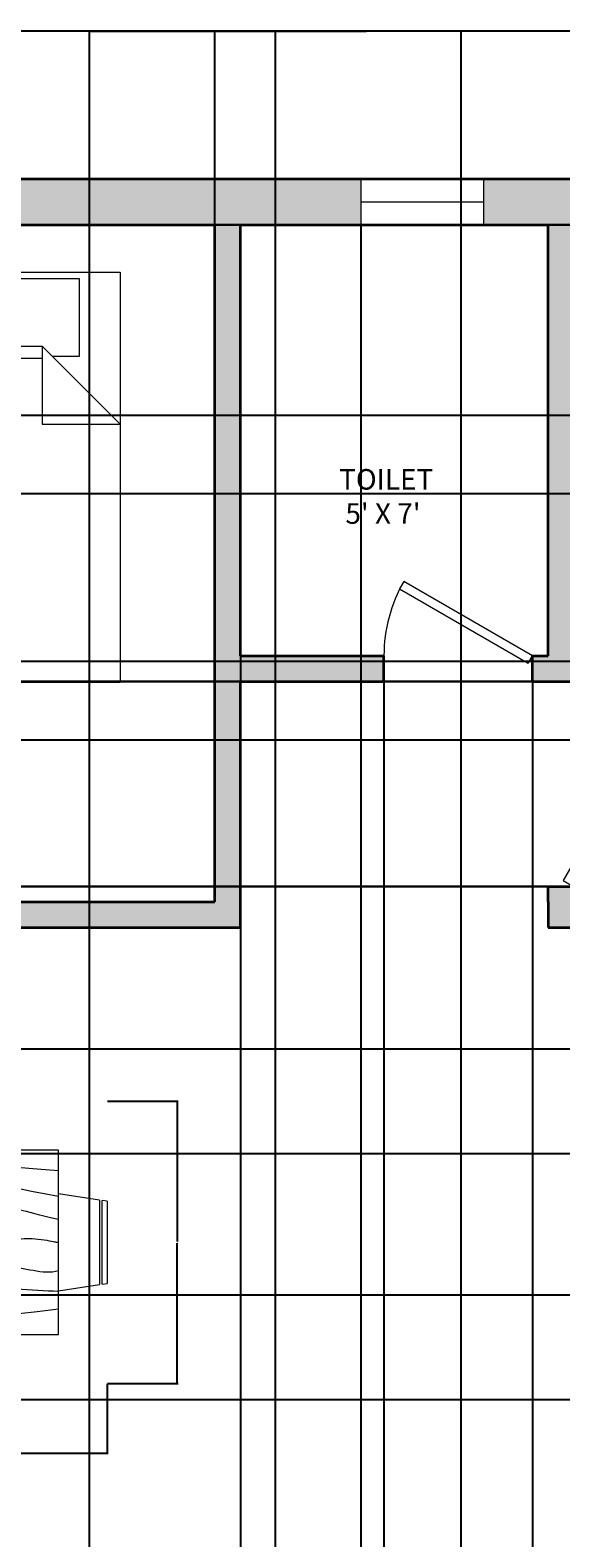
# Model space of a CAD drawing. Units: inches. Extents: x -28 to 649, y -11 to 509.
# Tile 6 of 7: x 346 to 450, y 215 to 509. Entities that reach past the tile are written whole.
import ezdxf

# ---------------------------------------------------------------- set-up
doc = ezdxf.new("R2010")
doc.units = ezdxf.units.IN
doc.header["$MEASUREMENT"] = 0
for name, color, linetype, lineweight in [('A-ANNO-DIMS', 2, 'Continuous', 18), ('A-AREA-IDEN', 18, 'Continuous', 18), ('A-WALL', 7, 'Continuous', 35), ('A-WALL-PATT', 251, 'Continuous', 13), ('doors', 40, 'Continuous', 20), ('furniture', 220, 'Continuous', 18), ('window', 30, 'Continuous', 18)]:
    doc.layers.add(name, color=color, linetype=linetype, lineweight=lineweight)
doc.styles.get("Standard").update_dxf_attribs({"font": 'arial.ttf'})
doc.dimstyles.get("Standard").update_dxf_attribs({"dimtxt": 0.18, "dimasz": 0.18, "dimexe": 0.18, "dimexo": 0.0625, "dimgap": 0.09, "dimtad": 0, "dimtih": 1, "dimtoh": 1, "dimdec": 4, "dimzin": 0, "dimdsep": 46, "dimtxsty": 'Standard', "dimcen": 0.09, "dimadec": 0, "dimazin": 0, "dimtfac": 1, "dimtdec": 4, "dimtofl": 0, "dimtmove": 0, "dimatfit": 3, "dimfxl": 1, "dimtolj": 1, "dimtzin": 0, "dimarcsym": 0})

# ---------------------------------------------------------------- blocks, each defined once
blk = doc.blocks.new('*U10')
for p, q in [((0, 0), (0, 100)), ((750, 0), (750, 100))]:
    blk.add_line(p, q)
blk.add_lwpolyline([(0, 0), (649.5, -375), (671.4, -337.1), (21.9, 37.9)], close=True)
blk.add_arc((0, 0), 750, 330, 0)
blk = doc.blocks.new('Dining Set - 36 x 72 in.')
for p, q in [((-22, 27.5), (-22.1562, 26.50042)), ((-5.8416, 26.5), (-22.1534, 26.5)), ((-22, 27.5), (-6, 27.5)), ((-5.8437, 26.49966), (-6, 27.5)), ((6, 27.5), (5.8438, 26.50042)), ((22.1584, 26.5), (5.8466, 26.5)), ((6, 27.5), (22, 27.5)), ((22.1563, 26.49966), (22, 27.5)), ((-22.2343, 26.00059), (-23.4847, 17.99762)), ((-22.2304, 26), (-5.7608, 26)), ((-4.5152, 17.99762), (-5.7655, 25.99926)), ((5.7657, 26.00059), (4.5153, 17.99762)), ((5.7696, 26), (22.2392, 26)), ((23.4848, 17.99762), (22.2345, 25.99926)), ((36, 18), (-36, 18)), ((-36, 18), (-36, -18)), ((36, -18), (36, 18)), ((-44.0006, 8.23428), (-35.9976, 9.48474)), ((44.0006, 8.23428), (35.9976, 9.48474)), ((-45.5, 8), (-44.5004, 8.15617)), ((-45.5, 8), (-45.5, -8)), ((-44.5, -8.15843), (-44.5, 8.15338)), ((-44, 8.23041), (-44, -8.23915)), ((44, 8.23041), (44, -8.23915)), ((44.5, -8.15843), (44.5, 8.15338)), ((45.5, 8), (44.5005, 8.15617)), ((45.5, 8), (45.5, -8)), ((-44.4997, -8.15631), (-45.5, -8)), ((-35.9976, -9.48476), (-43.9993, -8.2345)), ((35.9976, -9.48476), (43.9993, -8.2345)), ((44.4997, -8.15631), (45.5, -8)), ((-36, -18), (36, -18)), ((-22.2343, -26.0006), (-23.4847, -17.99762)), ((-4.5152, -17.99762), (-5.7655, -25.99928)), ((5.7657, -26.0006), (4.5153, -17.99762)), ((23.4848, -17.99762), (22.2345, -25.99928)), ((-22.2304, -26), (-5.7608, -26)), ((5.7696, -26), (22.2392, -26)), ((-22, -27.5), (-22.1562, -26.50044)), ((-5.8416, -26.5), (-22.1534, -26.5)), ((-22, -27.5), (-6, -27.5)), ((-5.8437, -26.49967), (-6, -27.5)), ((6, -27.5), (5.8438, -26.50044)), ((22.1584, -26.5), (5.8466, -26.5)), ((6, -27.5), (22, -27.5)), ((22.1563, -26.49967), (22, -27.5))]:
    blk.add_line(p, q)
for points in [[(-36, 15), (-31.1772, 14.97754), (-26.8079, 14.91406), (-22.8538, 14.81543), (-19.276, 14.6875), (-16.0362, 14.53613), (-13.0957, 14.36718), (-10.4159, 14.18652), (-7.9583, 14), (-5.6904, 13.81315), (-3.6035, 13.63021), (-1.6954, 13.45508), (0.0365, 13.29166), (1.5945, 13.14388), (2.9811, 13.01562), (4.1988, 12.9108), (5.25, 12.83333), (6.1393, 12.78613), (6.8802, 12.76823), (7.4883, 12.77767), (7.9792, 12.8125), (8.3685, 12.87077), (8.6719, 12.95052), (8.9049, 13.0498), (9.0833, 13.16666), (9.2205, 13.29899), (9.3216, 13.44401), (9.3895, 13.59879), (9.4271, 13.76041), (9.4373, 13.92594), (9.4232, 14.09245), (9.3875, 14.257), (9.3333, 14.41666), (9.2638, 14.56917), (9.1836, 14.71484), (9.0975, 14.85465), (9.0104, 14.98958), (8.9272, 15.1206), (8.8529, 15.2487), (8.7922, 15.37483), (8.75, 15.5), (8.7305, 15.62467), (8.7344, 15.74739), (8.7617, 15.86621), (8.8125, 15.97916), (8.8867, 16.08431), (8.9844, 16.17968), (9.1055, 16.26334), (9.25, 16.33333), (9.4189, 16.38802), (9.6172, 16.42708), (9.8506, 16.45052), (10.125, 16.45833), (10.4463, 16.45052), (10.8203, 16.42708), (11.2529, 16.38802), (11.75, 16.33333), (12.3184, 16.26318), (12.9694, 16.17838), (13.7151, 16.07991), (14.5677, 15.96875), (15.5395, 15.84586), (16.6426, 15.71224), (17.8893, 15.56884), (19.2917, 15.41666), (20.859, 15.25667), (22.5879, 15.08984), (24.4721, 14.91715), (26.5052, 14.73958), (28.6809, 14.5581), (30.9929, 14.3737), (33.4347, 14.18733), (36, 14)], [(-36, 10), (-28.9766, 10.14274), (-23.1725, 10.20442), (-18.4241, 10.19775), (-14.5677, 10.13541), (-11.4399, 10.03011), (-8.877, 9.89453), (-6.7154, 9.74137), (-4.7917, 9.58333), (-2.9698, 9.43082), (-1.2246, 9.28515), (0.4415, 9.14534), (2.026, 9.01041), (3.5266, 8.87939), (4.9408, 8.7513), (6.266, 8.62516), (7.5, 8.5), (8.6411, 8.37549), (9.6914, 8.2539), (10.6538, 8.13818), (11.5312, 8.03125), (12.3267, 7.93603), (13.043, 7.85547), (13.6831, 7.79248), (14.25, 7.75), (14.7471, 7.7303), (15.1797, 7.73307), (15.5537, 7.75732), (15.875, 7.80208), (16.1494, 7.86637), (16.3828, 7.94922), (16.5811, 8.04964), (16.75, 8.16666), (16.8944, 8.29915), (17.0143, 8.44531), (17.1089, 8.60319), (17.1771, 8.77083), (17.218, 8.94629), (17.2305, 9.1276), (17.2137, 9.31282), (17.1667, 9.5), (17.0895, 9.6875), (16.987, 9.875), (16.8649, 10.0625), (16.7292, 10.25), (16.5856, 10.4375), (16.4401, 10.625), (16.2985, 10.8125), (16.1667, 11), (16.05, 11.18733), (15.9518, 11.3737), (15.8752, 11.5581), (15.8229, 11.73958), (15.798, 11.91715), (15.8034, 12.08984), (15.842, 12.25667), (15.9167, 12.41666), (16.0295, 12.56836), (16.1784, 12.70833), (16.3605, 12.83268), (16.5729, 12.9375), (16.8127, 13.01888), (17.0768, 13.07291), (17.3625, 13.0957), (17.6667, 13.08333), (17.9894, 13.03312), (18.3418, 12.94726), (18.7382, 12.82918), (19.1927, 12.68229), (19.7195, 12.51001), (20.3327, 12.31575), (21.0465, 12.10294), (21.875, 11.875), (22.8357, 11.63354), (23.959, 11.37304), (25.2786, 11.08618), (26.8282, 10.76562), (28.6414, 10.40405), (30.752, 9.99414), (33.1936, 9.52856), (36, 9)], [(-36, 5.5), (-30.7157, 5.3348), (-26.069, 5.20963), (-21.9946, 5.11767), (-18.4271, 5.05208), (-15.3009, 5.00602), (-12.5508, 4.97265), (-10.1112, 4.94515), (-7.9167, 4.91666), (-5.909, 4.88167), (-4.0586, 4.83984), (-2.3429, 4.79215), (-0.7396, 4.73958), (0.7739, 4.6831), (2.22, 4.6237), (3.6213, 4.56233), (5, 4.5), (6.373, 4.43782), (7.7344, 4.3776), (9.0723, 4.32129), (10.375, 4.27083), (11.6309, 4.22819), (12.8281, 4.19531), (13.9551, 4.17415), (15, 4.16666), (15.954, 4.17448), (16.819, 4.19791), (17.6001, 4.23698), (18.3021, 4.29166), (18.9299, 4.36198), (19.4883, 4.44791), (19.9823, 4.54948), (20.4167, 4.66666), (20.7969, 4.79899), (21.1302, 4.94401), (21.4245, 5.09879), (21.6875, 5.26041), (21.9271, 5.42594), (22.1511, 5.59245), (22.3672, 5.757), (22.5834, 5.91666), (22.8065, 6.06868), (23.0404, 6.21093), (23.2879, 6.34147), (23.5521, 6.45833), (23.8358, 6.55957), (24.142, 6.64323), (24.4735, 6.70735), (24.8334, 6.75), (25.2235, 6.76969), (25.642, 6.76692), (26.0858, 6.74267), (26.5521, 6.69791), (27.0379, 6.63362), (27.5404, 6.55078), (28.0565, 6.45036), (28.5834, 6.33333), (29.1242, 6.19987), (29.7071, 6.04687), (30.3661, 5.87044), (31.1354, 5.66666), (32.0493, 5.43164), (33.142, 5.16146), (34.4475, 4.85221), (36, 4.5)], [(-36, -1), (-30.7915, -0.6591), (-26.0195, -0.38216), (-21.6519, -0.16284), (-17.6563, 0.00521), (-14.0005, 0.12833), (-10.6523, 0.21289), (-7.5796, 0.26522), (-4.75, 0.29166), (-2.134, 0.29793), (0.2878, 0.28711), (2.5317, 0.26163), (4.6146, 0.22396), (6.5529, 0.17651), (8.3633, 0.12174), (10.0623, 0.06209), (11.6667, 0), (13.1899, -0.06201), (14.6341, -0.1211), (15.9982, -0.17432), (17.2813, -0.21875), (18.4823, -0.25147), (19.6003, -0.26953), (20.6343, -0.27002), (21.5834, -0.25), (22.4481, -0.20768), (23.2357, -0.14584), (23.9549, -0.06836), (24.6146, 0.02083), (25.2235, 0.11784), (25.7904, 0.21875), (26.3241, 0.31966), (26.8334, 0.41666), (27.3265, 0.50618), (27.8099, 0.58593), (28.2894, 0.65397), (28.7709, 0.70833), (29.2601, 0.74707), (29.763, 0.76823), (30.2855, 0.76985), (30.8334, 0.75), (31.4088, 0.70784), (31.9994, 0.64713), (32.589, 0.57275), (33.1615, 0.48958), (33.7008, 0.4025), (34.1908, 0.3164), (34.6153, 0.23616), (34.9584, 0.16666), (35.2099, 0.11165), (35.3848, 0.07031), (35.504, 0.04069), (35.5886, 0.02083), (35.6594, 0.00879), (35.7377, 0.0026), (35.8442, 0.00032), (36, 0)], [(-36, -6.5), (-27.1843, -6.31267), (-20.084, -6.1263), (-14.469, -5.9419), (-10.1094, -5.76042), (-6.7752, -5.58285), (-4.2363, -5.41016), (-2.2629, -5.24333), (-0.625, -5.08334), (0.8708, -4.93099), (2.2715, -4.78646), (3.5872, -4.64974), (4.8281, -4.52084), (6.0046, -4.39974), (7.127, -4.28646), (8.2053, -4.18099), (9.25, -4.08334), (10.2705, -3.99382), (11.2734, -3.91407), (12.2647, -3.84603), (13.25, -3.79167), (14.2354, -3.75293), (15.2266, -3.73177), (16.2295, -3.73015), (17.25, -3.75), (18.2912, -3.79248), (19.3451, -3.85547), (20.4009, -3.93604), (21.4479, -4.03125), (22.4754, -4.13819), (23.4727, -4.25391), (24.4289, -4.37549), (25.3334, -4.5), (26.1785, -4.62492), (26.9694, -4.74935), (27.7145, -4.87281), (28.4219, -4.99479), (29.1, -5.11483), (29.7572, -5.23242), (30.4016, -5.34709), (31.0417, -5.45834), (31.6837, -5.56437), (32.3262, -5.65821), (32.9658, -5.73153), (33.599, -5.77604), (34.2224, -5.78345), (34.8327, -5.74545), (35.4264, -5.65373), (36, -5.5)], [(-36, -10), (-26.4022, -9.81299), (-18.4675, -9.62891), (-11.9839, -9.45069), (-6.7396, -9.28125), (-2.5226, -9.12354), (0.8789, -8.98047), (3.6769, -8.85498), (6.0833, -8.75), (8.2767, -8.66765), (10.3021, -8.60677), (12.1712, -8.56543), (13.8958, -8.54167), (15.4876, -8.53353), (16.9583, -8.53907), (18.3197, -8.55632), (19.5834, -8.58334), (20.7616, -8.61841), (21.8685, -8.66081), (22.9188, -8.71004), (23.9271, -8.76563), (24.9081, -8.82707), (25.8763, -8.89388), (26.8465, -8.96558), (27.8334, -9.04167), (28.8474, -9.12118), (29.8828, -9.20117), (30.93, -9.27824), (31.9792, -9.34896), (33.0205, -9.40991), (34.0443, -9.45768), (35.0407, -9.48885), (36, -9.5)], [(-36, -14.5), (-30.0881, -14.33513), (-25.0332, -14.21224), (-20.7312, -14.12647), (-17.0781, -14.07292), (-13.97, -14.04671), (-11.3027, -14.04297), (-8.9724, -14.05681), (-6.875, -14.08334), (-4.9224, -14.11833), (-3.0905, -14.16016), (-1.3709, -14.20785), (0.2448, -14.26042), (1.7647, -14.3169), (3.1973, -14.3763), (4.5507, -14.43767), (5.8333, -14.5), (7.0554, -14.5621), (8.235, -14.62175), (9.3922, -14.67652), (10.5469, -14.72396), (11.7192, -14.76164), (12.929, -14.78711), (14.1965, -14.79794), (15.5417, -14.79167), (16.9933, -14.76424), (18.6152, -14.70508), (20.4804, -14.60197), (22.6615, -14.44271), (25.2312, -14.21509), (28.2624, -13.9069), (31.8277, -13.50594), (36, -13)]]:
    blk.add_lwpolyline(points)
blk = doc.blocks.new('Bed - Queen')
for p, q in [((0, -80.00003), (0, 0)), ((0, 0), (59.99999, 0)), ((59.99999, 0), (59.99999, -80.00003)), ((7.99999, -1.2), (28.79998, -1.2)), ((7.99999, -14.4), (7.99999, -1.2)), ((28.79998, -1.2), (28.79998, -14.4)), ((31.19999, -1.2), (51.99999, -1.2)), ((31.19999, -14.4), (31.19999, -1.2)), ((51.99999, -1.2), (51.99999, -16.4)), ((0, -14.4), (44.8, -14.4)), ((59.99999, -29.6), (44.8, -14.4)), ((44.8, -14.4), (44.8, -29.6)), ((44.8, -16.8), (0, -16.8)), ((51.99999, -16.4), (46.79936, -16.4)), ((44.8, -29.6), (59.99999, -29.6)), ((59.99999, -80.00003), (0, -80.00003))]:
    blk.add_line(p, q)
blk = doc.blocks.new('WIN-24x9')
for p, q in [((0, 9), (0, 0)), ((24, 9), (0, 9)), ((0, 9), (0, 4.5)), ((24, 0), (24, 9)), ((0, 4.5), (24, 4.5)), ((0, 0), (24, 0))]:
    blk.add_line(p, q)
blk = doc.blocks.new('*D28')
at = {"layer": 'A-ANNO-DIMS', "color": 0, "lineweight": -2, "transparency": 16777216}
for p, q in [((270.49, 245), (270.49, 231.23)), ((361.49, 245), (361.49, 231.23)), ((270.67, 231.41), (315.04, 231.41)), ((361.31, 231.41), (316.94, 231.41))]:
    blk.add_line(p, q, dxfattribs=at)
at = {"layer": 'A-ANNO-DIMS', "color": 0, "transparency": 16777216}
for points in [[(270.67, 231.44), (270.67, 231.38), (270.49, 231.41)], [(361.31, 231.44), (361.31, 231.38), (361.49, 231.41)]]:
    blk.add_solid(points, dxfattribs=at)
at = {"layer": 'Defpoints', "color": 0, "transparency": 16777216}
for p in [(270.49, 245.06), (361.49, 245.06), (361.49, 231.41)]:
    blk.add_point(p, dxfattribs=at)
at = {"layer": 'A-ANNO-DIMS', "color": 0, "transparency": 16777216, "insert": (315.99, 231.41), "char_height": 0.18, "attachment_point": 5}
blk.add_mtext('\\A1;DINING SET 91', dxfattribs=at)
blk = doc.blocks.new('*D29')
at = {"layer": 'A-ANNO-DIMS', "color": 0, "lineweight": -2, "transparency": 16777216}
for p, q in [((361.55, 300.06), (375.32, 300.06)), ((375.14, 299.88), (375.14, 272.75)), ((375.14, 245.24), (375.14, 272.38)), ((361.55, 245.06), (375.32, 245.06))]:
    blk.add_line(p, q, dxfattribs=at)
at = {"layer": 'A-ANNO-DIMS', "color": 0, "transparency": 16777216}
for points in [[(375.11, 299.88), (375.17, 299.88), (375.14, 300.06)], [(375.11, 245.24), (375.17, 245.24), (375.14, 245.06)]]:
    blk.add_solid(points, dxfattribs=at)
at = {"layer": 'Defpoints', "color": 0, "transparency": 16777216}
for p in [(361.49, 300.06), (375.14, 300.06), (361.49, 245.06)]:
    blk.add_point(p, dxfattribs=at)
at = {"layer": 'A-ANNO-DIMS', "color": 0, "transparency": 16777216, "insert": (375.14, 272.56), "char_height": 0.18, "attachment_point": 5}
blk.add_mtext('\\A1;55', dxfattribs=at)
blk = doc.blocks.new('*D30')
at = {"layer": 'A-ANNO-DIMS', "color": 0, "lineweight": -2, "transparency": 16777216}
for p, q in [((27.45, 480), (27.45, 508.92)), ((27.63, 508.74), (315.16, 508.74)), ((603.27, 508.74), (315.74, 508.74)), ((603.45, 480), (603.45, 508.92))]:
    blk.add_line(p, q, dxfattribs=at)
at = {"layer": 'A-ANNO-DIMS', "color": 0, "transparency": 16777216}
for points in [[(27.63, 508.77), (27.63, 508.71), (27.45, 508.74)], [(603.27, 508.77), (603.27, 508.71), (603.45, 508.74)]]:
    blk.add_solid(points, dxfattribs=at)
at = {"layer": 'Defpoints', "color": 0, "transparency": 16777216}
for p in [(603.45, 508.74), (27.45, 479.94), (603.45, 479.94)]:
    blk.add_point(p, dxfattribs=at)
at = {"layer": 'A-ANNO-DIMS', "color": 0, "transparency": 16777216, "insert": (315.45, 508.74), "char_height": 0.18, "attachment_point": 5}
blk.add_mtext('\\A1;576', dxfattribs=at)
blk = doc.blocks.new('*D31')
at = {"layer": 'A-ANNO-DIMS', "color": 0, "lineweight": -2, "transparency": 16777216}
for p, q in [((603.51, 479.94), (632.43, 479.94)), ((632.25, 479.76), (632.25, 249.12)), ((632.25, 18.12), (632.25, 248.76)), ((346.51, 17.94), (632.43, 17.94))]:
    blk.add_line(p, q, dxfattribs=at)
at = {"layer": 'A-ANNO-DIMS', "color": 0, "transparency": 16777216}
for points in [[(632.22, 479.76), (632.28, 479.76), (632.25, 479.94)], [(632.22, 18.12), (632.28, 18.12), (632.25, 17.94)]]:
    blk.add_solid(points, dxfattribs=at)
at = {"layer": 'Defpoints', "color": 0, "transparency": 16777216}
for p in [(603.45, 479.94), (632.25, 479.94), (346.45, 17.94)]:
    blk.add_point(p, dxfattribs=at)
at = {"layer": 'A-ANNO-DIMS', "color": 0, "transparency": 16777216, "insert": (632.25, 248.94), "char_height": 0.18, "attachment_point": 5}
blk.add_mtext('\\A1;462', dxfattribs=at)
blk = doc.blocks.new('*D47')
at = {"layer": 'A-ANNO-DIMS', "color": 0, "lineweight": -2, "transparency": 16777216}
for p, q in [((387.45, 470.88), (387.45, -11.04)), ((410.91, 470.88), (410.91, -11.04)), ((387.63, -10.86), (398.79, -10.86)), ((410.73, -10.86), (399.58, -10.86))]:
    blk.add_line(p, q, dxfattribs=at)
at = {"layer": 'A-ANNO-DIMS', "color": 0, "transparency": 16777216}
for points in [[(387.63, -10.83), (387.63, -10.89), (387.45, -10.86)], [(410.73, -10.83), (410.73, -10.89), (410.91, -10.86)]]:
    blk.add_solid(points, dxfattribs=at)
at = {"layer": 'Defpoints', "color": 0, "transparency": 16777216}
for p in [(387.45, 470.94), (410.91, 470.94), (410.91, -10.86)]:
    blk.add_point(p, dxfattribs=at)
at = {"layer": 'A-ANNO-DIMS', "color": 0, "transparency": 16777216, "insert": (399.18, -10.86), "char_height": 0.18, "attachment_point": 5}
blk.add_mtext('\\A1;23.46', dxfattribs=at)
blk = doc.blocks.new('*D49')
at = {"layer": 'A-ANNO-DIMS', "color": 0, "lineweight": -2, "transparency": 16777216}
for p, q in [((36.51, 470.94), (632.43, 470.94)), ((632.25, 470.76), (632.25, 452.59)), ((632.25, 434.06), (632.25, 452.23)), ((36.51, 433.88), (632.43, 433.88))]:
    blk.add_line(p, q, dxfattribs=at)
at = {"layer": 'A-ANNO-DIMS', "color": 0, "transparency": 16777216}
for points in [[(632.22, 470.76), (632.28, 470.76), (632.25, 470.94)], [(632.22, 434.06), (632.28, 434.06), (632.25, 433.88)]]:
    blk.add_solid(points, dxfattribs=at)
at = {"layer": 'Defpoints', "color": 0, "transparency": 16777216}
for p in [(36.45, 470.94), (36.45, 433.88), (632.25, 433.88)]:
    blk.add_point(p, dxfattribs=at)
at = {"layer": 'A-ANNO-DIMS', "color": 0, "transparency": 16777216, "insert": (632.25, 452.41), "char_height": 0.18, "attachment_point": 5}
blk.add_mtext('\\A1;37.055', dxfattribs=at)
blk = doc.blocks.new('*D50')
at = {"layer": 'A-ANNO-DIMS', "color": 0, "lineweight": -2, "transparency": 16777216}
for p, q in [((594.39, 470.94), (-1.53, 470.94)), ((-1.35, 470.76), (-1.35, 444.89)), ((-1.35, 418.66), (-1.35, 444.53)), ((594.39, 418.48), (-1.53, 418.48))]:
    blk.add_line(p, q, dxfattribs=at)
at = {"layer": 'A-ANNO-DIMS', "color": 0, "transparency": 16777216}
for points in [[(-1.38, 470.76), (-1.32, 470.76), (-1.35, 470.94)], [(-1.38, 418.66), (-1.32, 418.66), (-1.35, 418.48)]]:
    blk.add_solid(points, dxfattribs=at)
at = {"layer": 'Defpoints', "color": 0, "transparency": 16777216}
for p in [(594.45, 470.94), (-1.35, 418.48), (594.45, 418.48)]:
    blk.add_point(p, dxfattribs=at)
at = {"layer": 'A-ANNO-DIMS', "color": 0, "transparency": 16777216, "insert": (-1.35, 444.71), "char_height": 0.18, "attachment_point": 5}
blk.add_mtext('\\A1;52.46', dxfattribs=at)
blk = doc.blocks.new('*D51')
at = {"layer": 'A-ANNO-DIMS', "color": 0, "lineweight": -2, "transparency": 16777216}
for p, q in [((594.39, 370.48), (-1.53, 370.48)), ((-1.35, 370.3), (-1.35, 340.55)), ((-1.35, 310.43), (-1.35, 340.19)), ((594.39, 310.25), (-1.53, 310.25))]:
    blk.add_line(p, q, dxfattribs=at)
at = {"layer": 'A-ANNO-DIMS', "color": 0, "transparency": 16777216}
for points in [[(-1.38, 370.3), (-1.32, 370.3), (-1.35, 370.48)], [(-1.38, 310.43), (-1.32, 310.43), (-1.35, 310.25)]]:
    blk.add_solid(points, dxfattribs=at)
at = {"layer": 'Defpoints', "color": 0, "transparency": 16777216}
for p in [(-1.35, 370.48), (594.45, 370.48), (594.45, 310.25)]:
    blk.add_point(p, dxfattribs=at)
at = {"layer": 'A-ANNO-DIMS', "color": 0, "transparency": 16777216, "insert": (-1.35, 340.37), "char_height": 0.18, "attachment_point": 5}
blk.add_mtext('\\A1;60.23', dxfattribs=at)
blk = doc.blocks.new('*D52')
at = {"layer": 'A-ANNO-DIMS', "color": 0, "lineweight": -2, "transparency": 16777216}
for p, q in [((594.39, 262.25), (-1.53, 262.25)), ((-1.35, 262.07), (-1.35, 206.61)), ((-1.35, 150.79), (-1.35, 206.25)), ((594.39, 150.61), (-1.53, 150.61))]:
    blk.add_line(p, q, dxfattribs=at)
at = {"layer": 'A-ANNO-DIMS', "color": 0, "transparency": 16777216}
for points in [[(-1.38, 262.07), (-1.32, 262.07), (-1.35, 262.25)], [(-1.38, 150.79), (-1.32, 150.79), (-1.35, 150.61)]]:
    blk.add_solid(points, dxfattribs=at)
at = {"layer": 'Defpoints', "color": 0, "transparency": 16777216}
for p in [(-1.35, 262.25), (594.45, 262.25), (594.45, 150.61)]:
    blk.add_point(p, dxfattribs=at)
at = {"layer": 'A-ANNO-DIMS', "color": 0, "transparency": 16777216, "insert": (-1.35, 206.43), "char_height": 0.18, "attachment_point": 5}
blk.add_mtext('\\A1;111.64', dxfattribs=at)
blk = doc.blocks.new('*D53')
at = {"layer": 'A-ANNO-DIMS', "color": 0, "lineweight": -2, "transparency": 16777216}
for p, q in [((36.51, 241.9), (632.43, 241.9)), ((632.25, 241.72), (632.25, 191.76)), ((632.25, 141.44), (632.25, 191.39)), ((36.51, 141.26), (632.43, 141.26))]:
    blk.add_line(p, q, dxfattribs=at)
at = {"layer": 'A-ANNO-DIMS', "color": 0, "transparency": 16777216}
for points in [[(632.22, 241.72), (632.28, 241.72), (632.25, 241.9)], [(632.22, 141.44), (632.28, 141.44), (632.25, 141.26)]]:
    blk.add_solid(points, dxfattribs=at)
at = {"layer": 'Defpoints', "color": 0, "transparency": 16777216}
for p in [(36.45, 241.9), (632.25, 241.9), (36.45, 141.26)]:
    blk.add_point(p, dxfattribs=at)
at = {"layer": 'A-ANNO-DIMS', "color": 0, "transparency": 16777216, "insert": (632.25, 191.58), "char_height": 0.18, "attachment_point": 5}
blk.add_mtext('\\A1;100.64', dxfattribs=at)
blk = doc.blocks.new('*D54')
at = {"layer": 'A-ANNO-DIMS', "color": 0, "lineweight": -2, "transparency": 16777216}
for p, q in [((36.51, 385.88), (632.43, 385.88)), ((632.25, 385.7), (632.25, 338.07)), ((632.25, 290.08), (632.25, 337.71)), ((36.51, 289.9), (632.43, 289.9))]:
    blk.add_line(p, q, dxfattribs=at)
at = {"layer": 'A-ANNO-DIMS', "color": 0, "transparency": 16777216}
for points in [[(632.22, 385.7), (632.28, 385.7), (632.25, 385.88)], [(632.22, 290.08), (632.28, 290.08), (632.25, 289.9)]]:
    blk.add_solid(points, dxfattribs=at)
at = {"layer": 'Defpoints', "color": 0, "transparency": 16777216}
for p in [(36.45, 385.88), (632.25, 385.88), (36.45, 289.9)]:
    blk.add_point(p, dxfattribs=at)
at = {"layer": 'A-ANNO-DIMS', "color": 0, "transparency": 16777216, "insert": (632.25, 337.89), "char_height": 0.18, "attachment_point": 5}
blk.add_mtext('\\A1;95.99', dxfattribs=at)
blk = doc.blocks.new('*D63')
at = {"layer": 'A-ANNO-DIMS', "color": 0, "lineweight": -2, "transparency": 16777216}
for p, q in [((415.45, 381.88), (415.45, -11.04)), ((444.45, 381.88), (444.45, -11.04)), ((415.63, -10.86), (429.73, -10.86)), ((444.27, -10.86), (430.17, -10.86))]:
    blk.add_line(p, q, dxfattribs=at)
at = {"layer": 'A-ANNO-DIMS', "color": 0, "transparency": 16777216}
for points in [[(415.63, -10.83), (415.63, -10.89), (415.45, -10.86)], [(444.27, -10.83), (444.27, -10.89), (444.45, -10.86)]]:
    blk.add_solid(points, dxfattribs=at)
at = {"layer": 'Defpoints', "color": 0, "transparency": 16777216}
for p in [(415.45, 381.94), (444.45, 381.94), (444.45, -10.86)]:
    blk.add_point(p, dxfattribs=at)
at = {"layer": 'A-ANNO-DIMS', "color": 0, "transparency": 16777216, "insert": (429.95, -10.86), "char_height": 0.18, "attachment_point": 5}
blk.add_mtext('\\A1;29', dxfattribs=at)
blk = doc.blocks.new('*D65')
at = {"layer": 'A-ANNO-DIMS', "color": 0, "lineweight": -2, "transparency": 16777216}
for p, q in [((185.51, 381.94), (632.43, 381.94)), ((632.25, 381.76), (632.25, 362.12)), ((632.25, 342.12), (632.25, 361.76)), ((185.51, 341.94), (632.43, 341.94))]:
    blk.add_line(p, q, dxfattribs=at)
at = {"layer": 'A-ANNO-DIMS', "color": 0, "transparency": 16777216}
for points in [[(632.22, 381.76), (632.28, 381.76), (632.25, 381.94)], [(632.22, 342.12), (632.28, 342.12), (632.25, 341.94)]]:
    blk.add_solid(points, dxfattribs=at)
at = {"layer": 'Defpoints', "color": 0, "transparency": 16777216}
for p in [(185.45, 381.94), (632.25, 381.94), (185.45, 341.94)]:
    blk.add_point(p, dxfattribs=at)
at = {"layer": 'A-ANNO-DIMS', "color": 0, "transparency": 16777216, "insert": (632.25, 361.94), "char_height": 0.18, "attachment_point": 5}
blk.add_mtext('\\A1;40', dxfattribs=at)
blk = doc.blocks.new('*D66')
at = {"layer": 'A-ANNO-DIMS', "color": 0, "lineweight": -2, "transparency": 16777216}
for p, q in [((447.05, 381.94), (-1.53, 381.94)), ((-1.35, 381.76), (-1.35, 362.12)), ((-1.35, 342.12), (-1.35, 361.76)), ((447.39, 341.94), (-1.53, 341.94))]:
    blk.add_line(p, q, dxfattribs=at)
at = {"layer": 'A-ANNO-DIMS', "color": 0, "transparency": 16777216}
for points in [[(-1.38, 381.76), (-1.32, 381.76), (-1.35, 381.94)], [(-1.38, 342.12), (-1.32, 342.12), (-1.35, 341.94)]]:
    blk.add_solid(points, dxfattribs=at)
at = {"layer": 'Defpoints', "color": 0, "transparency": 16777216}
for p in [(-1.35, 381.94), (447.12, 381.94), (447.45, 341.94)]:
    blk.add_point(p, dxfattribs=at)
at = {"layer": 'A-ANNO-DIMS', "color": 0, "transparency": 16777216, "insert": (-1.35, 361.94), "char_height": 0.18, "attachment_point": 5}
blk.add_mtext('\\A1;40', dxfattribs=at)
blk = doc.blocks.new('*D67')
at = {"layer": 'A-ANNO-DIMS', "color": 0, "lineweight": -2, "transparency": 16777216}
for p, q in [((250.45, 471), (250.45, 508.92)), ((250.63, 508.74), (316.17, 508.74)), ((382.27, 508.74), (316.73, 508.74)), ((382.45, 471), (382.45, 508.92))]:
    blk.add_line(p, q, dxfattribs=at)
at = {"layer": 'A-ANNO-DIMS', "color": 0, "transparency": 16777216}
for points in [[(250.63, 508.77), (250.63, 508.71), (250.45, 508.74)], [(382.27, 508.77), (382.27, 508.71), (382.45, 508.74)]]:
    blk.add_solid(points, dxfattribs=at)
at = {"layer": 'Defpoints', "color": 0, "transparency": 16777216}
for p in [(382.45, 508.74), (250.45, 470.94), (382.45, 470.94)]:
    blk.add_point(p, dxfattribs=at)
at = {"layer": 'A-ANNO-DIMS', "color": 0, "transparency": 16777216, "insert": (316.45, 508.74), "char_height": 0.18, "attachment_point": 5}
blk.add_mtext('\\A1;132', dxfattribs=at)
blk = doc.blocks.new('*D68')
at = {"layer": 'A-ANNO-DIMS', "color": 0, "lineweight": -2, "transparency": 16777216}
for p, q in [((358.05, 91.23), (358.05, 508.92)), ((358.23, 508.74), (411.94, 508.74)), ((466.55, 508.74), (412.85, 508.74)), ((466.73, 91.23), (466.73, 508.92))]:
    blk.add_line(p, q, dxfattribs=at)
at = {"layer": 'A-ANNO-DIMS', "color": 0, "transparency": 16777216}
for points in [[(358.23, 508.77), (358.23, 508.71), (358.05, 508.74)], [(466.55, 508.77), (466.55, 508.71), (466.73, 508.74)]]:
    blk.add_solid(points, dxfattribs=at)
at = {"layer": 'Defpoints', "color": 0, "transparency": 16777216}
for p in [(466.73, 508.74), (358.05, 91.17), (466.73, 91.17)]:
    blk.add_point(p, dxfattribs=at)
at = {"layer": 'A-ANNO-DIMS', "color": 0, "transparency": 16777216, "insert": (412.39, 508.74), "char_height": 0.18, "attachment_point": 5}
blk.add_mtext('\\A1;108.68', dxfattribs=at)
blk = doc.blocks.new('*D70')
at = {"layer": 'A-ANNO-DIMS', "color": 0, "lineweight": -2, "transparency": 16777216}
for p, q in [((394.28, 68.59), (394.28, 508.92)), ((394.46, 508.74), (412, 508.74)), ((430.33, 508.74), (412.79, 508.74)), ((430.51, 68.59), (430.51, 508.92))]:
    blk.add_line(p, q, dxfattribs=at)
at = {"layer": 'A-ANNO-DIMS', "color": 0, "transparency": 16777216}
for points in [[(394.46, 508.77), (394.46, 508.71), (394.28, 508.74)], [(430.33, 508.77), (430.33, 508.71), (430.51, 508.74)]]:
    blk.add_solid(points, dxfattribs=at)
at = {"layer": 'Defpoints', "color": 0, "transparency": 16777216}
for p in [(430.51, 508.74), (394.28, 68.53), (430.51, 68.53)]:
    blk.add_point(p, dxfattribs=at)
at = {"layer": 'A-ANNO-DIMS', "color": 0, "transparency": 16777216, "insert": (412.39, 508.74), "char_height": 0.18, "attachment_point": 5}
blk.add_mtext('\\A1;36.23', dxfattribs=at)

msp = doc.modelspace()

# ---------------------------------------------------------------- hatches: boundary and pattern name
at = {"layer": 'A-WALL-PATT'}
h = msp.add_hatch(color=256, dxfattribs=at)
h.dxf.hatch_style = 1
h.paths.add_polyline_path([(36.4499, 184.9382), (165.4499, 184.9382), (165.4499, 189.9382), (36.4499, 189.9382), (36.4499, 241.898), (27.4499, 241.898), (27.4499, 141.2558), (36.4499, 141.2558)])
h.paths.add_polyline_path([(36.4499, 385.8835), (27.4499, 385.8835), (27.4499, 289.898), (36.4499, 289.898)])
h.paths.add_polyline_path([(185.4499, 341.9382), (180.4499, 341.9382), (180.4499, 338.9382), (36.4499, 338.9382), (36.4499, 333.9382), (185.4499, 333.9382)])
h.paths.add_polyline_path([(36.4499, 470.9382), (79.2168, 470.9382), (79.2168, 479.9382), (27.4499, 479.9382), (27.4499, 433.8835), (36.4499, 433.8835)])
h.paths.add_polyline_path([(185.4499, 470.9382), (203.9104, 470.9382), (203.9104, 479.9382), (127.2168, 479.9382), (127.2168, 470.9382), (180.4499, 470.9382), (180.4499, 381.9382), (188.4499, 381.9382), (188.4499, 386.9382), (185.4499, 386.9382)])
h.paths.add_polyline_path([(292.4601, 479.9382), (227.9104, 479.9382), (227.9104, 470.9382), (245.4499, 470.9382), (245.4499, 386.9382), (217.4499, 386.9382), (217.4499, 381.9382), (245.4499, 381.9382), (245.4499, 338.9382), (245.4499, 333.9382), (251.5222, 333.9382), (251.5222, 338.9382), (250.4499, 338.9382), (250.4499, 470.9382), (292.4601, 470.9382)])
h.paths.add_polyline_path([(410.9121, 479.9382), (340.4601, 479.9382), (340.4601, 470.9382), (382.4499, 470.9382), (382.4499, 338.9382), (287.5222, 338.9382), (287.5222, 333.9382), (387.4499, 333.9382), (387.4499, 381.9382), (415.4499, 381.9382), (415.4499, 386.9382), (387.4499, 386.9382), (387.4499, 470.9382), (410.9121, 470.9382)])
h.paths.add_polyline_path([(497.0961, 479.9382), (434.9121, 479.9382), (434.9121, 470.9382), (447.4499, 470.9382), (447.4499, 386.9382), (444.4499, 386.9382), (444.4499, 381.9382), (452.4499, 381.9382), (452.4499, 470.9382), (497.0961, 470.9382)])
h.paths.add_polyline_path([(603.4499, 479.9382), (545.0961, 479.9382), (545.0961, 470.9382), (594.4499, 470.9382), (594.4499, 418.4819), (603.4499, 418.4819)])
h.paths.add_polyline_path([(603.4499, 370.4819), (594.4499, 370.4819), (594.4499, 338.9382), (452.4499, 338.9382), (452.4499, 341.9382), (447.4499, 341.9382), (447.4499, 338.9382), (447.4499, 333.9382), (594.4499, 333.9382), (594.4499, 310.2528), (603.4499, 310.2528)])
h.paths.add_polyline_path([(603.4499, 262.2528), (594.4499, 262.2528), (594.4499, 205.9382), (515.4499, 205.9382), (515.4499, 200.9382), (594.4499, 200.9382), (594.4499, 150.6102), (603.4499, 150.6102)])

# ---------------------------------------------------------------- linework, layer by layer
at = {"layer": 'A-WALL'}
for p, q in [((250.4499, 470.9382), (382.4499, 470.9382)), ((382.4499, 338.9382), (382.4499, 470.9382)), ((387.4499, 470.9382), (447.4499, 470.9382)), ((387.4499, 386.9382), (387.4499, 470.9382)), ((447.4499, 386.9382), (447.4499, 470.9382)), ((387.4499, 386.9382), (415.4499, 386.9382)), ((415.4499, 381.9382), (415.4499, 386.9382)), ((444.4499, 386.9382), (447.4499, 386.9382)), ((444.4499, 381.9382), (444.4499, 386.9382)), ((387.4499, 381.9382), (415.4499, 381.9382)), ((387.4499, 333.9382), (387.4499, 381.9382)), ((444.4499, 381.9382), (452.4499, 381.9382)), ((447.4499, 341.9382), (452.4499, 341.9382)), ((447.4499, 338.9382), (447.4499, 341.9382)), ((287.5222, 338.9382), (382.4499, 338.9382)), ((447.4499, 338.9382), (447.4499, 333.9382)), ((287.5222, 333.9382), (387.4499, 333.9382)), ((447.4499, 333.9382), (594.4499, 333.9382))]:
    msp.add_line(p, q, dxfattribs=at)
msp.add_lwpolyline([(209.4499, 47.9382), (27.4499, 47.9382), (27.4499, 479.9382), (603.4499, 479.9382), (603.4499, 47.9382), (269.4499, 47.9382)], dxfattribs=at)

# ---------------------------------------------------------------- block references
at = {"layer": 'doors'}
for p, xscale, yscale, zscale, rotation in [((444.4499, 386.9382), 0.0386666666666653, 0.0386666666666653, 0.0386666666666653, 180), ((452.4499, 341.9382), 0.0533333333333356, 0.0533333333333356, 0.0533333333333356, 90)]:
    msp.add_blockref('*U10', p, dxfattribs=dict(at, xscale=xscale, yscale=yscale, zscale=zscale, rotation=rotation))
at = {"layer": 'furniture'}
for name, p in [('Bed - Queen', (304.0136, 461.7144)), ('Dining Set - 36 x 72 in.', (315.9912, 272.5645))]:
    msp.add_blockref(name, p, dxfattribs=at)
at = {"layer": 'window'}
msp.add_blockref('WIN-24x9', (410.9121, 470.9382), dxfattribs=at)

# ---------------------------------------------------------------- texts
at = {"layer": 'A-AREA-IDEN', "insert": (406.7095, 423.3345), "char_height": 4, "attachment_point": 1}
msp.add_mtext_dynamic_manual_height_columns("TOILET\\P 5' X 7'", width=33.096465, gutter_width=1, heights=[0], dxfattribs=at)

# ---------------------------------------------------------------- dimensions: what is measured, and where the dimension line sits
at = {"layer": 'A-ANNO-DIMS'}
for base, p1, p2, override, picture, middle in [((603.4499, 508.7392), (27.4499, 479.9382), (603.4499, 479.9382), {"dimdec": 0, "dimlfac": 1, "dimrnd": 0, "dimzin": 0, "dimdsep": 46, "dimlunit": 2}, '*D30', (315.4499, 508.7392)), ((382.4499, 508.7392), (250.4499, 470.9382), (382.4499, 470.9382), {"dimdec": 0, "dimlfac": 1, "dimrnd": 0, "dimzin": 0, "dimdsep": 46, "dimlunit": 2}, '*D67', (316.4499, 508.7392)), ((466.7314, 508.7392), (358.0522, 91.1694), (466.7314, 91.1694), {"dimdec": 2, "dimlfac": 1, "dimrnd": 0, "dimzin": 0, "dimdsep": 46, "dimlunit": 2}, '*D68', (412.3918, 508.7392)), ((430.505, 508.7392), (394.2786, 68.5279), (430.505, 68.5279), {"dimdec": 2, "dimlfac": 1, "dimrnd": 0, "dimzin": 0, "dimdsep": 46, "dimlunit": 2}, '*D70', (412.3918, 508.7392)), ((410.9121, -10.8628), (387.4499, 470.9382), (410.9121, 470.9382), {"dimdec": 2, "dimlfac": 1, "dimrnd": 0, "dimzin": 0, "dimdsep": 46, "dimlunit": 2}, '*D47', (399.181, -10.8628)), ((444.4499, -10.8628), (415.4499, 381.9382), (444.4499, 381.9382), {"dimdec": 0, "dimlfac": 1, "dimrnd": 0, "dimzin": 0, "dimdsep": 46, "dimlunit": 2}, '*D63', (429.9499, -10.8628))]:
    dim = msp.add_linear_dim(base=base, p1=p1, p2=p2, dimstyle='Standard', override=override, dxfattribs=at)
    dim.commit()
    dim.dimension.update_dxf_attribs({"geometry": picture, "text_midpoint": middle})
for base, p1, p2, override, picture, middle in [((632.2509, 479.9382), (346.4499, 17.9382), (603.4499, 479.9382), {"dimdec": 0, "dimlfac": 1, "dimrnd": 0, "dimzin": 0, "dimdsep": 46, "dimlunit": 2}, '*D31', (632.2509, 248.9382)), ((-1.3511, 418.4819), (594.4499, 470.9382), (594.4499, 418.4819), {"dimdec": 2, "dimlfac": 1, "dimrnd": 0, "dimzin": 0, "dimdsep": 46, "dimlunit": 2}, '*D50', (-1.3511, 444.71)), ((632.2509, 433.8835), (36.4499, 470.9382), (36.4499, 433.8835), {"dimdec": 3, "dimlfac": 1, "dimrnd": 0, "dimzin": 0, "dimdsep": 46, "dimlunit": 2}, '*D49', (632.2509, 452.4109)), ((632.2509, 385.8835), (36.4499, 289.898), (36.4499, 385.8835), {"dimdec": 2, "dimlfac": 1, "dimrnd": 0, "dimzin": 0, "dimdsep": 46, "dimlunit": 2}, '*D54', (632.2509, 337.8907)), ((-1.3511, 381.9382), (447.4499, 341.9382), (447.1165, 381.9382), {"dimdec": 0, "dimlfac": 1, "dimrnd": 0, "dimzin": 0, "dimdsep": 46, "dimlunit": 2}, '*D66', (-1.3511, 361.9382)), ((632.2509, 381.9382), (185.4499, 341.9382), (185.4499, 381.9382), {"dimdec": 0, "dimlfac": 1, "dimrnd": 0, "dimzin": 0, "dimdsep": 46, "dimlunit": 2}, '*D65', (632.2509, 361.9382)), ((-1.3511, 370.4819), (594.4499, 310.2528), (594.4499, 370.4819), {"dimdec": 2, "dimlfac": 1, "dimrnd": 0, "dimzin": 0, "dimdsep": 46, "dimlunit": 2}, '*D51', (-1.3511, 340.3674)), ((375.1412, 300.0645), (361.4912, 245.0645), (361.4912, 300.0645), {"dimdec": 0, "dimlfac": 1, "dimrnd": 0, "dimzin": 0, "dimdsep": 46, "dimlunit": 2}, '*D29', (375.1412, 272.5645)), ((-1.3511, 262.2528), (594.4499, 150.6102), (594.4499, 262.2528), {"dimdec": 2, "dimlfac": 1, "dimrnd": 0, "dimzin": 0, "dimdsep": 46, "dimlunit": 2}, '*D52', (-1.3511, 206.4315)), ((632.2509, 241.898), (36.4499, 141.2558), (36.4499, 241.898), {"dimdec": 2, "dimlfac": 1, "dimrnd": 0, "dimzin": 0, "dimdsep": 46, "dimlunit": 2}, '*D53', (632.2509, 191.5769))]:
    dim = msp.add_linear_dim(base=base, p1=p1, p2=p2, angle=90, dimstyle='Standard', override=override, dxfattribs=at)
    dim.commit()
    dim.dimension.update_dxf_attribs({"geometry": picture, "text_midpoint": middle})
dim = msp.add_linear_dim(base=(361.4912, 231.4145), p1=(270.4912, 245.0645), p2=(361.4912, 245.0645), text='DINING SET <>', dimstyle='Standard', override={"dimdec": 0, "dimlfac": 1, "dimrnd": 0, "dimzin": 0, "dimdsep": 46, "dimlunit": 2}, dxfattribs=at)
dim.commit()
dim.dimension.update_dxf_attribs({"geometry": '*D28', "text_midpoint": (315.9912, 231.4145)})

doc.saveas('drawing.dxf')
